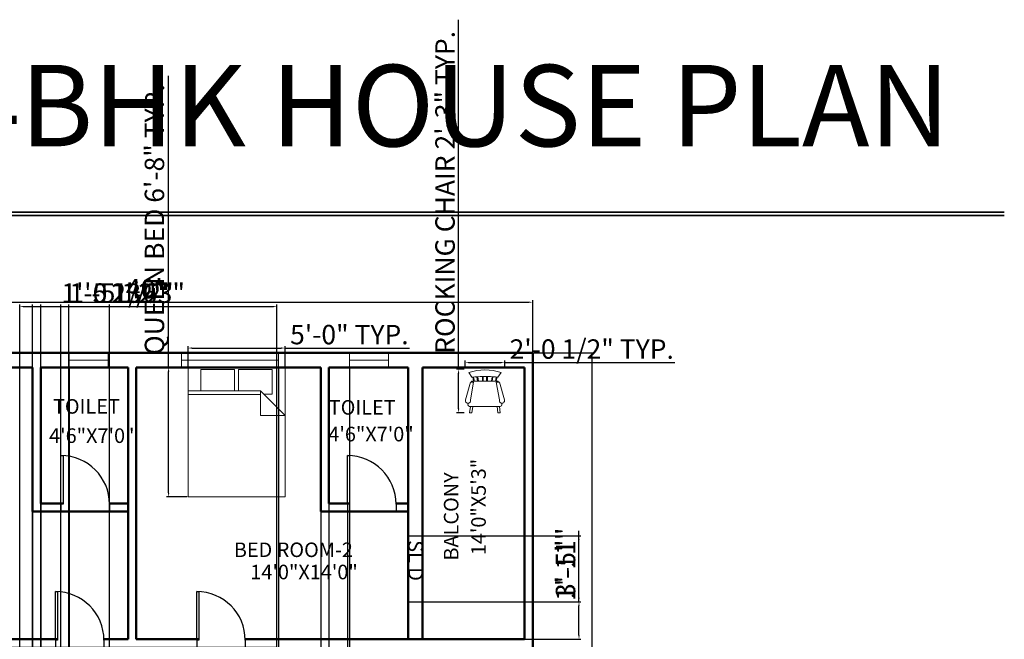
# Model space of a CAD drawing. Units: inches. Extents: x 2744 to 3775, y 2156 to 2963.
# Tile 4 of 4: x 3167 to 3775, y 2580 to 2963. Entities that reach past the tile are written whole.
import ezdxf

# ---------------------------------------------------------------- set-up
doc = ezdxf.new("R2010")
doc.units = ezdxf.units.IN
for name, color, linetype, lineweight in [('A-ANNO-DIMS', 2, 'Continuous', 18), ('A-ANNO-TEXT', 7, 'Continuous', 18), ('A-ANNO-TTLB', 210, 'Continuous', 35), ('A-AREA-IDEN', 7, 'Continuous', 25), ('A-DOOR', 3, 'Continuous', 25), ('A-FURN', 8, 'Continuous', 18), ('A-GLAZ', 4, 'Continuous', 18), ('A-WALL', 7, 'Continuous', 50)]:
    doc.layers.add(name, color=color, linetype=linetype, lineweight=lineweight)
doc.styles.get("Standard").update_dxf_attribs({"font": 'arial.ttf'})
doc.dimstyles.new('ISO-25', dxfattribs={"dimtxt": 12, "dimasz": 2.5, "dimexe": 1.25, "dimexo": 0.625, "dimtad": 1, "dimdec": 1, "dimlunit": 4, "dimtxsty": 'Standard', "dimcen": 2.5, "dimadec": 0, "dimazin": 0, "dimtfac": 1, "dimtdec": 1, "dimtmove": 0, "dimatfit": 3, "dimfxl": 1, "dimarcsym": 0})

# ---------------------------------------------------------------- blocks, each defined once
blk = doc.blocks.new('*U2')
for p, q in [((0, 0), (0, -6)), ((40, 0), (40, -6))]:
    blk.add_line(p, q)
blk.add_lwpolyline([(0, 0), (0, 40), (1.75, 40), (1.75, 0)], close=True)
blk.add_arc((0, 0), 40, 0, 90)
blk = doc.blocks.new('Bed - Queen')
for p, q in [((0, -80.00003), (0, 0)), ((0, 0), (59.99999, 0)), ((59.99999, 0), (59.99999, -80.00003)), ((7.99999, -1.2), (28.79998, -1.2)), ((7.99999, -14.4), (7.99999, -1.2)), ((28.79998, -1.2), (28.79998, -14.4)), ((31.19999, -1.2), (51.99999, -1.2)), ((31.19999, -14.4), (31.19999, -1.2)), ((51.99999, -1.2), (51.99999, -16.4)), ((0, -14.4), (44.8, -14.4)), ((44.8, -16.8), (0, -16.8)), ((59.99999, -29.6), (44.8, -14.4)), ((44.8, -14.4), (44.8, -29.6)), ((51.99999, -16.4), (46.79936, -16.4)), ((44.8, -29.6), (59.99999, -29.6)), ((59.99999, -80.00003), (0, -80.00003))]:
    blk.add_line(p, q)
blk = doc.blocks.new('Chair - Rocking')
for p, q in [((-8, -4.5), (-10, -1.5)), ((-7.5, -4.5), (-7, -7)), ((-6.5, -7), (-7.02225, -4.43)), ((-4.5, -7), (-4.96674, -4.19951)), ((-4, -7), (-4.40532, -4.16272)), ((-1.5, -4.05012), (-1.5, -7)), ((-1, -7), (-1, -4.05012)), ((1, -7), (1, -4.04655)), ((1.5, -4.05012), (1.5, -7)), ((4, -7), (4.40187, -4.18694)), ((4.5, -7), (4.96761, -4.19437)), ((6.5, -7), (7, -4.4057)), ((7.5, -4.5), (7, -7)), ((8, -4.5), (10, -1.5)), ((-9, -7.5), (-12, -18.49999)), ((-7, -7.5), (-9, -7.5)), ((-9, -18.49999), (-7, -7.5)), ((-8.23428, -6.99939), (-8.3093, -7.47958)), ((-8.23041, -7), (8.23915, -7)), ((7, -7.5), (9, -7.5)), ((9, -18.49999), (7, -7.5)), ((8.31071, -7.48854), (8.23449, -7.00073)), ((9, -7.5), (12, -18.49999)), ((-10.36644, -20.64523), (-10.5, -21.49999)), ((-9, -22.49999), (-9.5, -26.49999)), ((0, -22.49999), (-9.5, -22.49999)), ((-8, -26.49999), (-7.5, -22.49999)), ((0, -22.49999), (9.5, -22.49999)), ((8, -26.49999), (7.5, -22.49999)), ((9, -22.49999), (9.5, -26.49999)), ((10.5, -21.49999), (10.3575, -20.58798)), ((-9.5, -26.49999), (-8, -26.49999)), ((9.5, -26.49999), (8, -26.49999))]:
    blk.add_line(p, q)
for centre, radius, start, end in [((0, -34.08333), 34.08333, 72.93847, 107.0615), ((0, -68.25004), 64.25, 93.92211, 97.15267), ((0, -68.25004), 64.25, 82.84733, 93.92211), ((-10.5, -18.99999), 1.58114, 161.5651, 18.43495), ((-9.5, -21.49999), 1, 180, 270), ((10.5, -18.99999), 1.58114, 161.5651, 18.43495), ((9.5, -21.49999), 1, 270, 0)]:
    blk.add_arc(centre, radius, start, end)
blk = doc.blocks.new('*D14')
at = {"layer": 'A-ANNO-DIMS', "color": 0, "lineweight": -2, "transparency": 16777216}
for p, q in [((3003.92, 2757.73), (3003.92, 2789.67)), ((3006.42, 2788.42), (3481.42, 2788.42)), ((3483.92, 2757.73), (3483.92, 2789.67))]:
    blk.add_line(p, q, dxfattribs=at)
at = {"layer": 'A-ANNO-DIMS', "color": 0, "transparency": 16777216}
for points in [[(3006.42, 2788.84), (3006.42, 2788), (3003.92, 2788.42)], [(3481.42, 2788.84), (3481.42, 2788), (3483.92, 2788.42)]]:
    blk.add_solid(points, dxfattribs=at)
at = {"layer": 'Defpoints', "color": 0, "transparency": 16777216}
for p in [(3483.92, 2788.42), (3003.92, 2757.1), (3483.92, 2757.1)]:
    blk.add_point(p, dxfattribs=at)
at = {"layer": 'A-ANNO-DIMS', "color": 0, "transparency": 16777216, "insert": (3243.92, 2795.17), "char_height": 12, "attachment_point": 5}
blk.add_mtext("40'", dxfattribs=at)
blk = doc.blocks.new('*D15')
at = {"layer": 'A-ANNO-DIMS', "color": 0, "lineweight": -2, "transparency": 16777216}
for p, q in [((3484.55, 2757.1), (3521.77, 2757.1)), ((3520.52, 2754.6), (3520.52, 2255.6)), ((3484.55, 2253.1), (3521.77, 2253.1))]:
    blk.add_line(p, q, dxfattribs=at)
at = {"layer": 'A-ANNO-DIMS', "color": 0, "transparency": 16777216}
for points in [[(3520.11, 2754.6), (3520.94, 2754.6), (3520.52, 2757.1)], [(3520.11, 2255.6), (3520.94, 2255.6), (3520.52, 2253.1)]]:
    blk.add_solid(points, dxfattribs=at)
at = {"layer": 'Defpoints', "color": 0, "transparency": 16777216}
for p in [(3483.92, 2757.1), (3483.92, 2253.1), (3520.52, 2253.1)]:
    blk.add_point(p, dxfattribs=at)
at = {"layer": 'A-ANNO-DIMS', "color": 0, "transparency": 16777216, "insert": (3513.88, 2505.1), "char_height": 12, "attachment_point": 5, "rotation": 90}
blk.add_mtext("42'", dxfattribs=at)
blk = doc.blocks.new('WIN-60IN')
blk.add_line((0, 4.5), (60, 4.5))
blk.add_lwpolyline([(0, 9), (60, 9), (60, 0), (0, 0)], close=True)
blk = doc.blocks.new('WIN-24IN')
blk.add_line((0, 4.5), (24, 4.5))
blk.add_lwpolyline([(0, 9), (24, 9), (24, 0), (0, 0)], close=True)
blk = doc.blocks.new('*D22')
at = {"layer": 'A-ANNO-DIMS', "color": 0, "lineweight": -2, "transparency": 16777216}
for p, q in [((3258.94, 2748.1), (3258.94, 2928.38)), ((3270.32, 2748.1), (3257.69, 2748.1)), ((3258.94, 2670.6), (3258.94, 2745.6)), ((3270.32, 2668.1), (3257.69, 2668.1))]:
    blk.add_line(p, q, dxfattribs=at)
at = {"layer": 'A-ANNO-DIMS', "color": 0, "transparency": 16777216}
for points in [[(3258.53, 2745.6), (3259.36, 2745.6), (3258.94, 2748.1)], [(3258.53, 2670.6), (3259.36, 2670.6), (3258.94, 2668.1)]]:
    blk.add_solid(points, dxfattribs=at)
at = {"layer": 'Defpoints', "color": 0, "transparency": 16777216}
for p in [(3258.94, 2748.1), (3270.94, 2748.1), (3270.94, 2668.1)]:
    blk.add_point(p, dxfattribs=at)
at = {"layer": 'A-ANNO-DIMS', "color": 0, "transparency": 16777216, "insert": (3251.74, 2839.49), "char_height": 12, "attachment_point": 5, "rotation": 90}
blk.add_mtext('QUEEN BED 6\'-8" TYP.', dxfattribs=at)
blk = doc.blocks.new('*D23')
at = {"layer": 'A-ANNO-DIMS', "color": 0, "lineweight": -2, "transparency": 16777216}
for p, q in [((3270.94, 2748.73), (3270.94, 2761.35)), ((3273.44, 2760.1), (3328.44, 2760.1)), ((3330.94, 2748.73), (3330.94, 2761.35)), ((3330.94, 2760.1), (3407.84, 2760.1))]:
    blk.add_line(p, q, dxfattribs=at)
at = {"layer": 'A-ANNO-DIMS', "color": 0, "transparency": 16777216}
for points in [[(3273.44, 2760.52), (3273.44, 2759.69), (3270.94, 2760.1)], [(3328.44, 2760.52), (3328.44, 2759.69), (3330.94, 2760.1)]]:
    blk.add_solid(points, dxfattribs=at)
at = {"layer": 'Defpoints', "color": 0, "transparency": 16777216}
for p in [(3330.94, 2760.1), (3270.94, 2748.1), (3330.94, 2748.1)]:
    blk.add_point(p, dxfattribs=at)
at = {"layer": 'A-ANNO-DIMS', "color": 0, "transparency": 16777216, "insert": (3370.64, 2766.86), "char_height": 12, "attachment_point": 5}
blk.add_mtext('5\'-0" TYP.', dxfattribs=at)
blk = doc.blocks.new('*D24')
at = {"layer": 'A-ANNO-DIMS', "color": 0, "lineweight": -2, "transparency": 16777216}
for p, q in [((3438.13, 2747.04), (3438.13, 2963.03)), ((3441.56, 2747.04), (3436.88, 2747.04)), ((3438.13, 2722.54), (3438.13, 2744.54)), ((3441.56, 2720.04), (3436.88, 2720.04))]:
    blk.add_line(p, q, dxfattribs=at)
at = {"layer": 'A-ANNO-DIMS', "color": 0, "transparency": 16777216}
for points in [[(3437.72, 2744.54), (3438.55, 2744.54), (3438.13, 2747.04)], [(3437.72, 2722.54), (3438.55, 2722.54), (3438.13, 2720.04)]]:
    blk.add_solid(points, dxfattribs=at)
at = {"layer": 'Defpoints', "color": 0, "transparency": 16777216}
for p in [(3438.13, 2747.04), (3442.18, 2747.04), (3442.18, 2720.04)]:
    blk.add_point(p, dxfattribs=at)
at = {"layer": 'A-ANNO-DIMS', "color": 0, "transparency": 16777216, "insert": (3431.3, 2856.28), "char_height": 12, "attachment_point": 5, "rotation": 90}
blk.add_mtext('ROCKING CHAIR 2\'-3" TYP.', dxfattribs=at)
blk = doc.blocks.new('*D25')
at = {"layer": 'A-ANNO-DIMS', "color": 0, "lineweight": -2, "transparency": 16777216}
for p, q in [((3442.18, 2747.67), (3442.18, 2752.34)), ((3444.68, 2751.09), (3464.12, 2751.09)), ((3466.62, 2747.67), (3466.62, 2752.34)), ((3466.62, 2751.09), (3571.68, 2751.09))]:
    blk.add_line(p, q, dxfattribs=at)
at = {"layer": 'A-ANNO-DIMS', "color": 0, "transparency": 16777216}
for points in [[(3444.68, 2751.51), (3444.68, 2750.68), (3442.18, 2751.09)], [(3464.12, 2751.51), (3464.12, 2750.68), (3466.62, 2751.09)]]:
    blk.add_solid(points, dxfattribs=at)
at = {"layer": 'Defpoints', "color": 0, "transparency": 16777216}
for p in [(3466.62, 2751.09), (3442.18, 2747.04), (3466.62, 2747.04)]:
    blk.add_point(p, dxfattribs=at)
at = {"layer": 'A-ANNO-DIMS', "color": 0, "transparency": 16777216, "insert": (3520.4, 2757.92), "char_height": 12, "attachment_point": 5}
blk.add_mtext('2\'-0 1/2" TYP.', dxfattribs=at)
blk = doc.blocks.new('*D32')
at = {"layer": 'A-ANNO-DIMS', "color": 0, "lineweight": -2, "transparency": 16777216}
for p, q in [((3212.07, 2547.39), (3076.42, 2547.39)), ((3212.07, 2541.68), (3212.07, 2548.64)), ((3251.79, 2547.39), (3214.57, 2547.39)), ((3254.29, 2541.68), (3254.29, 2548.64))]:
    blk.add_line(p, q, dxfattribs=at)
at = {"layer": 'A-ANNO-DIMS', "color": 0, "transparency": 16777216}
for points in [[(3214.57, 2547.81), (3214.57, 2546.97), (3212.07, 2547.39)], [(3251.79, 2547.81), (3251.79, 2546.97), (3254.29, 2547.39)]]:
    blk.add_solid(points, dxfattribs=at)
at = {"layer": 'Defpoints', "color": 0, "transparency": 16777216}
for p in [(3212.07, 2547.39), (3212.07, 2541.06), (3254.29, 2541.06)]:
    blk.add_point(p, dxfattribs=at)
at = {"layer": 'A-ANNO-DIMS', "color": 0, "transparency": 16777216, "insert": (3143, 2554.22), "char_height": 12, "attachment_point": 5}
blk.add_mtext('DINING SET 3\'-6"', dxfattribs=at)
blk = doc.blocks.new('*D34')
at = {"layer": 'A-ANNO-DIMS', "color": 0, "lineweight": -2, "transparency": 16777216}
for p, q in [((3145.86, 2747.48), (3145.86, 2223.25)), ((3174.92, 2747.48), (3174.92, 2223.25)), ((3148.36, 2224.5), (3172.42, 2224.5)), ((3174.92, 2224.5), (3210.78, 2224.5))]:
    blk.add_line(p, q, dxfattribs=at)
at = {"layer": 'A-ANNO-DIMS', "color": 0, "transparency": 16777216}
for points in [[(3148.36, 2224.92), (3148.36, 2224.09), (3145.86, 2224.5)], [(3172.42, 2224.92), (3172.42, 2224.09), (3174.92, 2224.5)]]:
    blk.add_solid(points, dxfattribs=at)
at = {"layer": 'Defpoints', "color": 0, "transparency": 16777216}
for p in [(3145.86, 2748.1), (3174.92, 2748.1), (3174.92, 2224.5)]:
    blk.add_point(p, dxfattribs=at)
at = {"layer": 'A-ANNO-DIMS', "color": 0, "transparency": 16777216, "insert": (3194.1, 2231.26), "char_height": 12, "attachment_point": 5}
blk.add_mtext('2\'-5"', dxfattribs=at)
blk = doc.blocks.new('*D35')
at = {"layer": 'A-ANNO-DIMS', "color": 0, "lineweight": -2, "transparency": 16777216}
for p, q in [((3179.92, 2747.48), (3179.92, 2223.25)), ((3197.52, 2747.48), (3197.52, 2223.25)), ((3182.42, 2224.5), (3195.02, 2224.5)), ((3197.52, 2224.5), (3260.01, 2224.5))]:
    blk.add_line(p, q, dxfattribs=at)
at = {"layer": 'A-ANNO-DIMS', "color": 0, "transparency": 16777216}
for points in [[(3182.42, 2224.92), (3182.42, 2224.09), (3179.92, 2224.5)], [(3195.02, 2224.92), (3195.02, 2224.09), (3197.52, 2224.5)]]:
    blk.add_solid(points, dxfattribs=at)
at = {"layer": 'Defpoints', "color": 0, "transparency": 16777216}
for p in [(3179.92, 2748.1), (3197.52, 2748.1), (3197.52, 2224.5)]:
    blk.add_point(p, dxfattribs=at)
at = {"layer": 'A-ANNO-DIMS', "color": 0, "transparency": 16777216, "insert": (3230.02, 2231.33), "char_height": 12, "attachment_point": 5}
blk.add_mtext('1\'-5 1/2"', dxfattribs=at)
blk = doc.blocks.new('*D36')
at = {"layer": 'A-ANNO-DIMS', "color": 0, "lineweight": -2, "transparency": 16777216}
for p, q in [((3326.88, 2747.48), (3326.88, 2223.25)), ((3352.92, 2747.48), (3352.92, 2223.25)), ((3329.38, 2224.5), (3350.42, 2224.5)), ((3352.92, 2224.5), (3388.78, 2224.5))]:
    blk.add_line(p, q, dxfattribs=at)
at = {"layer": 'A-ANNO-DIMS', "color": 0, "transparency": 16777216}
for points in [[(3329.38, 2224.92), (3329.38, 2224.09), (3326.88, 2224.5)], [(3350.42, 2224.92), (3350.42, 2224.09), (3352.92, 2224.5)]]:
    blk.add_solid(points, dxfattribs=at)
at = {"layer": 'Defpoints', "color": 0, "transparency": 16777216}
for p in [(3326.88, 2748.1), (3352.92, 2748.1), (3352.92, 2224.5)]:
    blk.add_point(p, dxfattribs=at)
at = {"layer": 'A-ANNO-DIMS', "color": 0, "transparency": 16777216, "insert": (3372.1, 2231.15), "char_height": 12, "attachment_point": 5}
blk.add_mtext('2\'-2"', dxfattribs=at)
blk = doc.blocks.new('*D37')
at = {"layer": 'A-ANNO-DIMS', "color": 0, "lineweight": -2, "transparency": 16777216}
for p, q in [((3357.92, 2747.48), (3357.92, 2223.25)), ((3370.78, 2747.48), (3370.78, 2223.25)), ((3360.42, 2224.5), (3368.28, 2224.5)), ((3370.78, 2224.5), (3405.3, 2224.5))]:
    blk.add_line(p, q, dxfattribs=at)
at = {"layer": 'A-ANNO-DIMS', "color": 0, "transparency": 16777216}
for points in [[(3360.42, 2224.92), (3360.42, 2224.09), (3357.92, 2224.5)], [(3368.28, 2224.92), (3368.28, 2224.09), (3370.78, 2224.5)]]:
    blk.add_solid(points, dxfattribs=at)
at = {"layer": 'Defpoints', "color": 0, "transparency": 16777216}
for p in [(3357.92, 2748.1), (3370.78, 2748.1), (3370.78, 2224.5)]:
    blk.add_point(p, dxfattribs=at)
at = {"layer": 'A-ANNO-DIMS', "color": 0, "transparency": 16777216, "insert": (3389.29, 2231.15), "char_height": 12, "attachment_point": 5}
blk.add_mtext('1\'-1"', dxfattribs=at)
blk = doc.blocks.new('*D39')
at = {"layer": 'A-ANNO-DIMS', "color": 0, "lineweight": -2, "transparency": 16777216}
for p, q in [((3179.92, 2262.73), (3179.92, 2786.95)), ((3197.36, 2262.73), (3197.36, 2786.95)), ((3182.42, 2785.7), (3194.86, 2785.7)), ((3197.36, 2785.7), (3259.85, 2785.7))]:
    blk.add_line(p, q, dxfattribs=at)
at = {"layer": 'A-ANNO-DIMS', "color": 0, "transparency": 16777216}
for points in [[(3182.42, 2786.12), (3182.42, 2785.29), (3179.92, 2785.7)], [(3194.86, 2786.12), (3194.86, 2785.29), (3197.36, 2785.7)]]:
    blk.add_solid(points, dxfattribs=at)
at = {"layer": 'Defpoints', "color": 0, "transparency": 16777216}
for p in [(3197.36, 2785.7), (3179.92, 2262.1), (3197.36, 2262.1)]:
    blk.add_point(p, dxfattribs=at)
at = {"layer": 'A-ANNO-DIMS', "color": 0, "transparency": 16777216, "insert": (3229.85, 2792.53), "char_height": 12, "attachment_point": 5}
blk.add_mtext('1\'-5 1/2"', dxfattribs=at)
blk = doc.blocks.new('*D49')
at = {"layer": 'A-ANNO-DIMS', "color": 0, "lineweight": -2, "transparency": 16777216}
for p, q in [((3416.55, 2644.12), (3513.77, 2644.12)), ((3512.52, 2605.83), (3512.52, 2641.62)), ((3416.55, 2603.33), (3513.77, 2603.33))]:
    blk.add_line(p, q, dxfattribs=at)
at = {"layer": 'A-ANNO-DIMS', "color": 0, "transparency": 16777216}
for points in [[(3512.11, 2641.62), (3512.94, 2641.62), (3512.52, 2644.12)], [(3512.11, 2605.83), (3512.94, 2605.83), (3512.52, 2603.33)]]:
    blk.add_solid(points, dxfattribs=at)
at = {"layer": 'Defpoints', "color": 0, "transparency": 16777216}
for p in [(3415.92, 2644.12), (3512.52, 2644.12), (3415.92, 2603.33)]:
    blk.add_point(p, dxfattribs=at)
at = {"layer": 'A-ANNO-DIMS', "color": 0, "transparency": 16777216, "insert": (3505.77, 2623.72), "char_height": 12, "attachment_point": 5, "rotation": 90}
blk.add_mtext('3\'-5"', dxfattribs=at)
blk = doc.blocks.new('*D52')
at = {"layer": 'A-ANNO-DIMS', "color": 0, "lineweight": -2, "transparency": 16777216}
for p, q in [((3166.92, 2435.73), (3166.92, 2786.95)), ((3325.92, 2430.73), (3325.92, 2786.95)), ((3169.42, 2785.7), (3323.42, 2785.7))]:
    blk.add_line(p, q, dxfattribs=at)
at = {"layer": 'A-ANNO-DIMS', "color": 0, "transparency": 16777216}
for points in [[(3169.42, 2786.12), (3169.42, 2785.29), (3166.92, 2785.7)], [(3323.42, 2786.12), (3323.42, 2785.29), (3325.92, 2785.7)]]:
    blk.add_solid(points, dxfattribs=at)
at = {"layer": 'Defpoints', "color": 0, "transparency": 16777216}
for p in [(3325.92, 2785.7), (3166.92, 2435.1), (3325.92, 2430.1)]:
    blk.add_point(p, dxfattribs=at)
at = {"layer": 'A-ANNO-DIMS', "color": 0, "transparency": 16777216, "insert": (3246.42, 2792.46), "char_height": 12, "attachment_point": 5}
blk.add_mtext('13\'-3"', dxfattribs=at)
blk = doc.blocks.new('*D53')
at = {"layer": 'A-ANNO-DIMS', "color": 0, "lineweight": -2, "transparency": 16777216}
for p, q in [((2975.32, 2575.1), (2975.32, 2638.71)), ((3325.3, 2575.1), (2974.07, 2575.1)), ((2975.32, 2535.1), (2975.32, 2572.6)), ((3325.3, 2532.6), (2974.07, 2532.6))]:
    blk.add_line(p, q, dxfattribs=at)
at = {"layer": 'A-ANNO-DIMS', "color": 0, "transparency": 16777216}
for points in [[(2974.91, 2572.6), (2975.74, 2572.6), (2975.32, 2575.1)], [(2974.91, 2535.1), (2975.74, 2535.1), (2975.32, 2532.6)]]:
    blk.add_solid(points, dxfattribs=at)
at = {"layer": 'Defpoints', "color": 0, "transparency": 16777216}
for p in [(2975.32, 2575.1), (3325.92, 2575.1), (3325.92, 2532.6)]:
    blk.add_point(p, dxfattribs=at)
at = {"layer": 'A-ANNO-DIMS', "color": 0, "transparency": 16777216, "insert": (2968.49, 2608.16), "char_height": 12, "attachment_point": 5, "rotation": 90}
blk.add_mtext('3\'-6 1/2"', dxfattribs=at)
blk = doc.blocks.new('*D57')
at = {"layer": 'A-ANNO-DIMS', "color": 0, "lineweight": -2, "transparency": 16777216}
for p, q in [((3192.43, 2351.37), (3192.43, 2786.95)), ((3222.43, 2351.37), (3222.43, 2786.95)), ((3194.93, 2785.7), (3219.93, 2785.7)), ((3222.43, 2785.7), (3258.28, 2785.7))]:
    blk.add_line(p, q, dxfattribs=at)
at = {"layer": 'A-ANNO-DIMS', "color": 0, "transparency": 16777216}
for points in [[(3194.93, 2786.12), (3194.93, 2785.29), (3192.43, 2785.7)], [(3219.93, 2786.12), (3219.93, 2785.29), (3222.43, 2785.7)]]:
    blk.add_solid(points, dxfattribs=at)
at = {"layer": 'Defpoints', "color": 0, "transparency": 16777216}
for p in [(3222.43, 2785.7), (3192.43, 2350.75), (3222.43, 2350.75)]:
    blk.add_point(p, dxfattribs=at)
at = {"layer": 'A-ANNO-DIMS', "color": 0, "transparency": 16777216, "insert": (3241.6, 2792.46), "char_height": 12, "attachment_point": 5}
blk.add_mtext('2\'-6"', dxfattribs=at)
blk = doc.blocks.new('*D58')
at = {"layer": 'A-ANNO-DIMS', "color": 0, "lineweight": -2, "transparency": 16777216}
for p, q in [((3174.92, 2351.73), (3174.92, 2786.95)), ((3192.43, 2351.37), (3192.43, 2786.95)), ((3177.42, 2785.7), (3189.93, 2785.7)), ((3192.43, 2785.7), (3254.91, 2785.7))]:
    blk.add_line(p, q, dxfattribs=at)
at = {"layer": 'A-ANNO-DIMS', "color": 0, "transparency": 16777216}
for points in [[(3177.42, 2786.12), (3177.42, 2785.29), (3174.92, 2785.7)], [(3189.93, 2786.12), (3189.93, 2785.29), (3192.43, 2785.7)]]:
    blk.add_solid(points, dxfattribs=at)
at = {"layer": 'Defpoints', "color": 0, "transparency": 16777216}
for p in [(3192.43, 2785.7), (3174.92, 2351.1), (3192.43, 2350.75)]:
    blk.add_point(p, dxfattribs=at)
at = {"layer": 'A-ANNO-DIMS', "color": 0, "transparency": 16777216, "insert": (3224.92, 2792.53), "char_height": 12, "attachment_point": 5}
blk.add_mtext('1\'-5 1/2"', dxfattribs=at)
blk = doc.blocks.new('*D61')
at = {"layer": 'A-ANNO-DIMS', "color": 0, "lineweight": -2, "transparency": 16777216}
for p, q in [((3512.52, 2603.33), (3512.52, 2647.17)), ((3416.55, 2603.33), (3513.77, 2603.33)), ((3512.52, 2582.6), (3512.52, 2600.83)), ((3416.55, 2580.1), (3513.77, 2580.1))]:
    blk.add_line(p, q, dxfattribs=at)
at = {"layer": 'A-ANNO-DIMS', "color": 0, "transparency": 16777216}
for points in [[(3512.11, 2600.83), (3512.94, 2600.83), (3512.52, 2603.33)], [(3512.11, 2582.6), (3512.94, 2582.6), (3512.52, 2580.1)]]:
    blk.add_solid(points, dxfattribs=at)
at = {"layer": 'Defpoints', "color": 0, "transparency": 16777216}
for p in [(3415.92, 2603.33), (3512.52, 2603.33), (3415.92, 2580.1)]:
    blk.add_point(p, dxfattribs=at)
at = {"layer": 'A-ANNO-DIMS', "color": 0, "transparency": 16777216, "insert": (3505.87, 2626.5), "char_height": 12, "attachment_point": 5, "rotation": 90}
blk.add_mtext('1\'-11"', dxfattribs=at)
blk = doc.blocks.new('*D64')
at = {"layer": 'A-ANNO-DIMS', "color": 0, "lineweight": -2, "transparency": 16777216}
for p, q in [((3179.92, 2664.73), (3179.92, 2786.95)), ((3192.43, 2664.23), (3192.43, 2786.95)), ((3182.42, 2785.7), (3189.93, 2785.7)), ((3192.43, 2785.7), (3254.91, 2785.7))]:
    blk.add_line(p, q, dxfattribs=at)
at = {"layer": 'A-ANNO-DIMS', "color": 0, "transparency": 16777216}
for points in [[(3182.42, 2786.12), (3182.42, 2785.29), (3179.92, 2785.7)], [(3189.93, 2786.12), (3189.93, 2785.29), (3192.43, 2785.7)]]:
    blk.add_solid(points, dxfattribs=at)
at = {"layer": 'Defpoints', "color": 0, "transparency": 16777216}
for p in [(3192.43, 2785.7), (3179.92, 2664.1), (3192.43, 2663.6)]:
    blk.add_point(p, dxfattribs=at)
at = {"layer": 'A-ANNO-DIMS', "color": 0, "transparency": 16777216, "insert": (3224.92, 2792.53), "char_height": 12, "attachment_point": 5}
blk.add_mtext('1\'-0 1/2"', dxfattribs=at)
blk = doc.blocks.new('*D65')
at = {"layer": 'A-ANNO-DIMS', "color": 0, "lineweight": -2, "transparency": 16777216}
for p, q in [((3352.92, 2658.48), (3352.92, 2223.25)), ((3369.47, 2658.48), (3369.47, 2223.25)), ((3355.42, 2224.5), (3366.97, 2224.5)), ((3369.47, 2224.5), (3431.96, 2224.5))]:
    blk.add_line(p, q, dxfattribs=at)
at = {"layer": 'A-ANNO-DIMS', "color": 0, "transparency": 16777216}
for points in [[(3355.42, 2224.92), (3355.42, 2224.09), (3352.92, 2224.5)], [(3366.97, 2224.92), (3366.97, 2224.09), (3369.47, 2224.5)]]:
    blk.add_solid(points, dxfattribs=at)
at = {"layer": 'Defpoints', "color": 0, "transparency": 16777216}
for p in [(3352.92, 2659.1), (3369.47, 2659.1), (3369.47, 2224.5)]:
    blk.add_point(p, dxfattribs=at)
at = {"layer": 'A-ANNO-DIMS', "color": 0, "transparency": 16777216, "insert": (3401.97, 2231.33), "char_height": 12, "attachment_point": 5}
blk.add_mtext('1\'-4 1/2"', dxfattribs=at)

msp = doc.modelspace()

# ---------------------------------------------------------------- linework, layer by layer
at = {"layer": 'A-ANNO-TTLB'}
for p, q in [((2752.61, 2844.08), (3775.35, 2844.08)), ((2752.61, 2842.08), (3775.35, 2842.08))]:
    msp.add_line(p, q, dxfattribs=at)
at = {"layer": 'A-DOOR'}
for p, q in [((3406.92, 2644.12), (3415.92, 2644.12)), ((3406.92, 2603.33), (3415.92, 2603.33))]:
    msp.add_line(p, q, dxfattribs=at)
at = {"layer": 'A-WALL'}
for p, q in [((3003.92, 2757.1), (3483.92, 2757.1)), ((3483.92, 2757.1), (3483.92, 2253.1)), ((3065.92, 2748.1), (3174.92, 2748.1)), ((3065.92, 2748.1), (3174.92, 2748.1)), ((3174.92, 2659.1), (3174.92, 2748.1)), ((3179.92, 2664.1), (3179.92, 2748.1)), ((3179.92, 2748.1), (3233.92, 2748.1)), ((3179.92, 2748.1), (3233.92, 2748.1)), ((3233.92, 2580.1), (3233.92, 2748.1)), ((3238.92, 2580.1), (3238.92, 2748.1)), ((3238.92, 2748.1), (3352.92, 2748.1)), ((3238.92, 2748.1), (3352.92, 2748.1)), ((3352.92, 2659.1), (3352.92, 2748.1)), ((3357.92, 2664.1), (3357.92, 2748.1)), ((3357.92, 2748.1), (3406.92, 2748.1)), ((3357.92, 2748.1), (3406.92, 2748.1)), ((3406.92, 2580.1), (3406.92, 2748.1)), ((3415.92, 2580.1), (3415.92, 2748.1)), ((3415.92, 2748.1), (3478.92, 2748.1)), ((3478.92, 2748.1), (3478.92, 2580.1)), ((3174.92, 2659.1), (3233.92, 2659.1)), ((3179.92, 2664.1), (3193.74, 2664.1)), ((3222.42, 2664.1), (3233.92, 2664.1)), ((3352.92, 2659.1), (3406.92, 2659.1)), ((3357.92, 2664.1), (3370.79, 2664.1)), ((3399.47, 2664.1), (3406.92, 2664.1)), ((3065.92, 2580.1), (3190.29, 2580.1)), ((3218.97, 2580.1), (3233.92, 2580.1)), ((3238.92, 2580.1), (3277.61, 2580.1)), ((3306.3, 2580.1), (3406.92, 2580.1)), ((3406.92, 2580.1), (3478.92, 2580.1))]:
    msp.add_line(p, q, dxfattribs=at)

# ---------------------------------------------------------------- block references
at = {"layer": 'A-DOOR', "xscale": 0.75, "yscale": 0.75, "zscale": 0.75}
for p in [(3192.43, 2663.6), (3369.47, 2663.6), (3188.98, 2579.6), (3276.3, 2579.6)]:
    msp.add_blockref('*U2', p, dxfattribs=at)
at = {"layer": 'A-FURN'}
for name, p in [('Bed - Queen', (3270.94, 2748.1)), ('Chair - Rocking', (3454.4, 2746.54))]:
    msp.add_blockref(name, p, dxfattribs=at)
at = {"layer": 'A-GLAZ'}
for name, p in [('WIN-24IN', (3197.52, 2748.1)), ('WIN-60IN', (3266.88, 2748.1)), ('WIN-24IN', (3370.78, 2748.1))]:
    msp.add_blockref(name, p, dxfattribs=at)

# ---------------------------------------------------------------- texts
at = {"layer": 'A-ANNO-TEXT'}
msp.add_text('SL D', height=9, rotation=270, dxfattribs=at).set_placement((3407.08, 2641.36))
at = {"layer": 'A-ANNO-TTLB'}
msp.add_text('40\'0"X42\'0" 4BHK HOUSE PLAN', height=50.3636, dxfattribs=at).set_placement((2742.18, 2884.73))
at = {"layer": 'A-AREA-IDEN'}
for s, p in [('TOILET', (3187.49, 2719.54)), ('TOILET', (3357.92, 2718.94)), ('4\'6"X7\'0"', (3185.09, 2701.47)), ('4\'6"X7\'0"', (3357.64, 2702.44)), ('BED ROOM-2', (3299.25, 2630.93)), ('14\'0"X14\'0"', (3309.45, 2617.19))]:
    msp.add_text(s, height=9, dxfattribs=at).set_placement(p)
for s, p in [('14\'0"X5\'3"', (3454.95, 2632.08)), ('BALCONY', (3438.03, 2628.78))]:
    msp.add_text(s, height=9, rotation=90, dxfattribs=at).set_placement(p)

# ---------------------------------------------------------------- dimensions: what is measured, and where the dimension line sits
at = {"layer": 'A-ANNO-DIMS'}
for base, p1, p2, angle, text, picture, middle in [((3438.13, 2747.04), (3442.18, 2720.04), (3442.18, 2747.04), 90, 'ROCKING CHAIR <> TYP.', '*D24', (3431.3, 2856.28)), ((3258.94, 2748.1), (3270.94, 2668.1), (3270.94, 2748.1), 90, 'QUEEN BED <> TYP.', '*D22', (3251.74, 2839.49)), ((3212.07, 2547.39), (3254.29, 2541.06), (3212.07, 2541.06), 180, 'DINING SET <>', '*D32', (3143, 2554.22))]:
    dim = msp.add_linear_dim(base=base, p1=p1, p2=p2, angle=angle, text=text, dimstyle='ISO-25', override={"dimdec": 1, "dimlfac": 1, "dimrnd": 0, "dimzin": 1, "dimdsep": 46, "dimlunit": 4, "dimfrac": 2}, dxfattribs=at)
    dim.commit()
    dim.dimension.update_dxf_attribs({"geometry": picture, "text_midpoint": middle})
for base, p1, p2, override, picture, middle in [((3192.43, 2785.7), (3174.92, 2351.1), (3192.43, 2350.75), {"dimdec": 1, "dimlfac": 1, "dimrnd": 0, "dimzin": 1, "dimdsep": 46, "dimlunit": 4, "dimfrac": 2}, '*D58', (3224.92, 2792.53)), ((3197.36, 2785.7), (3179.92, 2262.1), (3197.36, 2262.1), {"dimdec": 1, "dimlfac": 1, "dimrnd": 0, "dimzin": 1, "dimdsep": 46, "dimlunit": 4, "dimfrac": 2}, '*D39', (3229.85, 2792.53)), ((3192.43, 2785.7), (3179.92, 2664.1), (3192.43, 2663.6), {"dimdec": 1, "dimlfac": 1, "dimrnd": 0, "dimzin": 1, "dimdsep": 46, "dimlunit": 4, "dimfrac": 2}, '*D64', (3224.92, 2792.53)), ((3483.92, 2788.42), (3003.92, 2757.1), (3483.92, 2757.1), {"dimclrd": 0, "dimclre": 0, "dimclrt": 0}, '*D14', (3243.92, 2795.17)), ((3325.92, 2785.7), (3166.92, 2435.1), (3325.92, 2430.1), {"dimdec": 1, "dimlfac": 1, "dimrnd": 0, "dimzin": 1, "dimdsep": 46, "dimlunit": 4, "dimfrac": 2}, '*D52', (3246.42, 2792.46)), ((3222.43, 2785.7), (3192.43, 2350.75), (3222.43, 2350.75), {"dimdec": 1, "dimlfac": 1, "dimrnd": 0, "dimzin": 1, "dimdsep": 46, "dimlunit": 4, "dimfrac": 2}, '*D57', (3241.6, 2792.46)), ((3174.92, 2224.5), (3145.86, 2748.1), (3174.92, 2748.1), {"dimdec": 1, "dimlfac": 1, "dimrnd": 0, "dimzin": 1, "dimdsep": 46, "dimlunit": 4, "dimfrac": 2}, '*D34', (3194.1, 2231.26)), ((3197.52, 2224.5), (3179.92, 2748.1), (3197.52, 2748.1), {"dimdec": 1, "dimlfac": 1, "dimrnd": 0, "dimzin": 1, "dimdsep": 46, "dimlunit": 4, "dimfrac": 2}, '*D35', (3230.02, 2231.33)), ((3352.92, 2224.5), (3326.88, 2748.1), (3352.92, 2748.1), {"dimdec": 1, "dimlfac": 1, "dimrnd": 0, "dimzin": 1, "dimdsep": 46, "dimlunit": 4, "dimfrac": 2}, '*D36', (3372.1, 2231.15)), ((3370.78, 2224.5), (3357.92, 2748.1), (3370.78, 2748.1), {"dimdec": 1, "dimlfac": 1, "dimrnd": 0, "dimzin": 1, "dimdsep": 46, "dimlunit": 4, "dimfrac": 2}, '*D37', (3389.29, 2231.15)), ((3369.4749, 2224.505), (3352.9224, 2659.105), (3369.4749, 2659.105), {"dimdec": 1, "dimlfac": 1, "dimrnd": 0, "dimzin": 1, "dimdsep": 46, "dimlunit": 4, "dimfrac": 2}, '*D65', (3401.9655, 2231.3346))]:
    dim = msp.add_linear_dim(base=base, p1=p1, p2=p2, dimstyle='ISO-25', override=override, dxfattribs=at)
    dim.commit()
    dim.dimension.update_dxf_attribs({"geometry": picture, "text_midpoint": middle})
for base, p1, p2, picture, middle in [((3330.94, 2760.1), (3270.94, 2748.1), (3330.94, 2748.1), '*D23', (3370.64, 2766.86)), ((3466.62, 2751.09), (3442.18, 2747.04), (3466.62, 2747.04), '*D25', (3520.4, 2757.92))]:
    dim = msp.add_linear_dim(base=base, p1=p1, p2=p2, text='<> TYP.', dimstyle='ISO-25', override={"dimdec": 1, "dimlfac": 1, "dimrnd": 0, "dimzin": 1, "dimdsep": 46, "dimlunit": 4, "dimfrac": 2}, dxfattribs=at)
    dim.commit()
    dim.dimension.update_dxf_attribs({"geometry": picture, "text_midpoint": middle})
for base, p1, p2, override, picture, middle in [((3520.52, 2253.1), (3483.92, 2757.1), (3483.92, 2253.1), {"dimclrd": 0, "dimclre": 0, "dimclrt": 0}, '*D15', (3513.88, 2505.1)), ((3512.52, 2603.33), (3415.92, 2580.1), (3415.92, 2603.33), {"dimdec": 1, "dimlfac": 1, "dimrnd": 0, "dimzin": 1, "dimdsep": 46, "dimlunit": 4, "dimfrac": 2}, '*D61', (3505.87, 2626.5)), ((3512.52, 2644.12), (3415.92, 2603.33), (3415.92, 2644.12), {"dimdec": 1, "dimlfac": 1, "dimrnd": 0, "dimzin": 1, "dimdsep": 46, "dimlunit": 4, "dimfrac": 2}, '*D49', (3505.77, 2623.72)), ((2975.32, 2575.1), (3325.92, 2532.6), (3325.92, 2575.1), {"dimdec": 1, "dimlfac": 1, "dimrnd": 0, "dimzin": 1, "dimdsep": 46, "dimlunit": 4, "dimfrac": 2}, '*D53', (2968.49, 2608.16))]:
    dim = msp.add_linear_dim(base=base, p1=p1, p2=p2, angle=90, dimstyle='ISO-25', override=override, dxfattribs=at)
    dim.commit()
    dim.dimension.update_dxf_attribs({"geometry": picture, "text_midpoint": middle})

doc.saveas('drawing.dxf')
